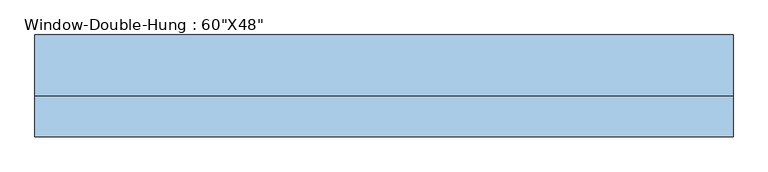
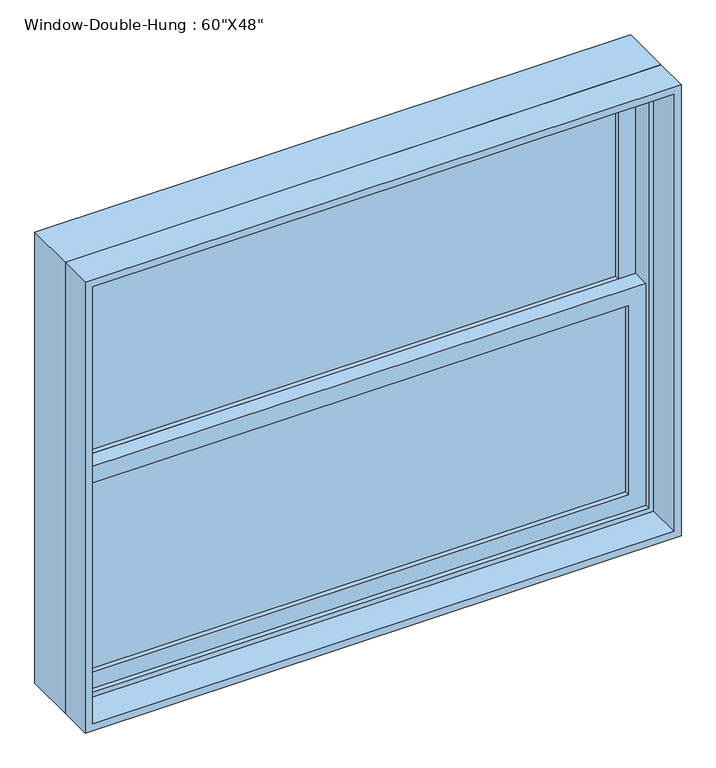
"""IFC4 building model written with IfcOpenShell, lengths in millimetres: window geometry."""

from ifc_helpers import new_model, si_unit, frame, origin, place, context, project, spatial, polyline, outline, extrude, source, transform, mapped, element, save


def window_d7d477dd(model_context):
    return source(origin(), model_context, "Body", "SweptSolid", [
        extrude(outline(polyline([(685.8, 31.75), (685.8, 25.4), (-685.8, 25.4), (-685.8, 31.75), (685.8, 31.75)])), frame((0.0, 0.0, 990.6), z_axis=(0.0, 0.0, 1.0), x_axis=(1.0, 0.0, 0.0)), (0.0, 0.0, 1.0), 511.175),
        extrude(outline(polyline([(-685.8, 19.05), (685.8, 19.05), (685.8, 12.7), (-685.8, 12.7), (-685.8, 19.05)])), frame((0.0, 0.0, 990.6), z_axis=(0.0, 0.0, 1.0), x_axis=(1.0, 0.0, 0.0)), (0.0, 0.0, 1.0), 511.175),
        extrude(outline(polyline([(685.8, 76.2), (685.8, 69.85), (-685.8, 69.85), (-685.8, 76.2), (685.8, 76.2)])), frame((0.0, 0.0, 1546.225), z_axis=(0.0, 0.0, 1.0), x_axis=(1.0, 0.0, 0.0)), (0.0, 0.0, 1.0), 511.175),
        extrude(outline(polyline([(-685.8, 63.5), (685.8, 63.5), (685.8, 57.15), (-685.8, 57.15), (-685.8, 63.5)])), frame((0.0, 0.0, 1546.225), z_axis=(0.0, 0.0, 1.0), x_axis=(1.0, 0.0, 0.0)), (0.0, 0.0, 1.0), 511.175),
        extrude(outline(polyline([(1546.225, -730.25), (946.15, -730.25), (946.15, 730.25), (1546.225, 730.25), (1546.225, -730.25)]), holes=[polyline([(1501.775, 685.8), (990.6, 685.8), (990.6, -685.8), (1501.775, -685.8), (1501.775, 685.8)])]), frame((0.0, 0.0, 0.0), z_axis=(0.0, 1.0, 0.0), x_axis=(0.0, 0.0, 1.0)), (0.0, 0.0, 1.0), 44.45),
        extrude(outline(polyline([(2101.85, -730.25), (1501.775, -730.25), (1501.775, 730.25), (2101.85, 730.25), (2101.85, -730.25)]), holes=[polyline([(2057.4, 685.8), (1546.225, 685.8), (1546.225, -685.8), (2057.4, -685.8), (2057.4, 685.8)])]), frame((0.0, 44.45, 0.0), z_axis=(0.0, 1.0, 0.0), x_axis=(0.0, 0.0, 1.0)), (0.0, 0.0, 1.0), 44.45),
        extrude(outline(polyline([(2133.6, -762.0), (914.4, -762.0), (914.4, 762.0), (2133.6, 762.0), (2133.6, -762.0)]), holes=[polyline([(2101.85, 730.25), (946.15, 730.25), (946.15, -730.25), (2101.85, -730.25), (2101.85, 730.25)])]), frame((0.0, -12.7, 0.0), z_axis=(0.0, 1.0, 0.0), x_axis=(0.0, 0.0, 1.0)), (0.0, 0.0, 1.0), 133.35),
        extrude(outline(polyline([(2133.6, 762.0), (2133.6, -762.0), (914.4, -762.0), (914.4, 762.0), (2133.6, 762.0)]), holes=[polyline([(2114.55, 742.95), (933.45, 742.95), (933.45, -742.95), (2114.55, -742.95), (2114.55, 742.95)])]), frame((0.0, -101.6, 0.0), z_axis=(0.0, 1.0, 0.0), x_axis=(0.0, 0.0, 1.0)), (0.0, 0.0, 1.0), 88.9),
    ])


if __name__ == "__main__":
    model = new_model("IFC4")
    model_context = context("Model", 3, world=origin())
    ifc_project = project(units=[si_unit("LENGTHUNIT", "METRE", prefix="MILLI")], contexts=[model_context])
    site = spatial("IfcSite", under=ifc_project)
    building = spatial("IfcBuilding", under=site)
    placement = place(None, origin())
    window_shape = window_d7d477dd(model_context)
    element("IfcWindow", 1, ObjectType="Window-Double-Hung : 60\"X48\"", at=placement, inside=building, context=model_context, shape_type="MappedRepresentation", body=[
        mapped(window_shape, transform((0.0, 0.0, 0.0), x_axis=(1.0, 0.0, 0.0), y_axis=(0.0, 1.0, 0.0), z_axis=(0.0, 0.0, 1.0))),
    ])
    save(model, "model.ifc")

# Revit data of these elements
# Type "Window-Double-Hung : 60\"X48\""
#   Type Mark = "18"
#   Fire Rating = "0.5h"
#   Construction Type Id = "DG-DR"
#   Assembly Code = "B2020100"
#   Analytic Construction = "Double glazing - domestic"
#   Wall Thickness [instance default] = 0' - 6"
#   Window Inset [instance default] = 0' - 0"
#   Visual Light Transmittance = 0.81
#   Thermal Resistance (R) = 1.8146 (h·ft²·°F)/BTU
#   Solar Heat Gain Coefficient = 0.76
#   Muntin Width = 4' - 6"
#   Muntin Height = 1' - 8 1/8"
#   Interior Wall Closure [instance default] = 0' - 1 1/2"
#   Rough Width = 5' - 0 1/2"
#   Rough Height = 4' - 0 1/2"
#   Frame Extension [instance default] = 0' - 1 1/4"
#   Exterior Wall Closure [instance default] = 0' - 0 1/2"
#   Extension Jamb [instance default] = 0' - 1 1/2"
#   Heat Transfer Coefficient (U) = 0.5511 BTU/(h·ft²·°F)
#   Height = 4' - 0"
#   Width = 5' - 0"
#   Top Muntin Visibility = yes
#   Indicator Visibility [instance default] = yes
#   Extension Jamb Visibility [instance default] = yes
#   Interior Trim Visibility [instance default] = yes
#   Exterior Trim Visibility [instance default] = yes
#   Define Thermal Properties by = 1
#   Bottom Muntin Visibility = yes
#   Muntin Pattern = Muntin Pattern_2x2 : Muntin Pattern_2x2
#   Interior Trim Material = Wood - Stained
#   Interior Trim = Trim-Window-Interior-Flat : Picture Frame
#   Exterior Trim Material = Clad - White
#   Exterior Trim = Trim-Window-Exterior-Flat : with Sill
#   Glass Panel Material = Glass
#   Exterior Frame Material = Clad - White
#   Interior Frame Material = Wood - Stained
#   Wall Closure = (empty or 0)
# Element 1 (IfcWindow, "Window-Double-Hung : 60\"X48\"")
#   Wall Thickness = 0' - 8"
#   Extension Jamb = 0' - 3 1/2"
#   Materials on its faces: "Wood - Stained", "Glass", "Clad - White"
# Materials
#   "Wood - Stained": class "Wood", colour RGB 224 178 126, transparency 0, Cost = 0
#   "Clad - White": class "Wood", colour RGB 242 242 238, transparency 0, Cost = 0
#   "Glass": class "Glass", colour RGB 0 128 192, transparency 0.75, Description = "Soda Lime Glass", Cost = 0
